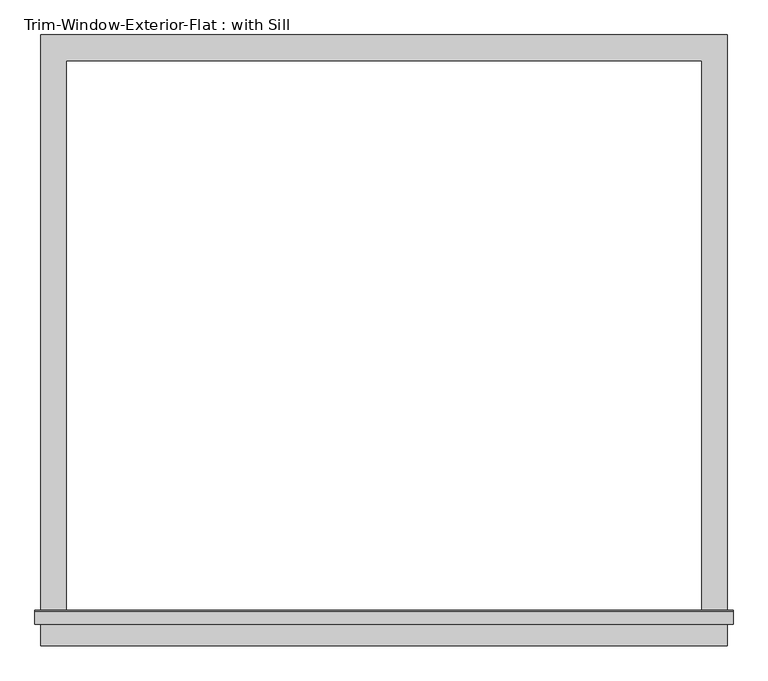
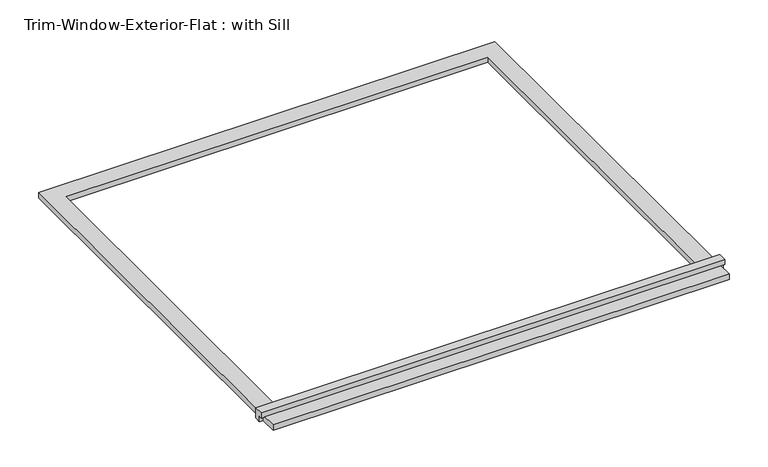
"""IFC4 building model written with IfcOpenShell, lengths in millimetres: proxy geometry, Trim-Window-Exterior-Flat : with Sill."""

from ifc_helpers import new_model, si_unit, frame, origin, origin_with_axes, place, context, project, spatial, polyline, outline, extrude, source, transform, mapped, element, save


def trim_window_exterior_flat_with_sill_cb7cc766(model_context):
    return source(origin(), model_context, "Body", "SweptSolid", [
        extrude(outline(polyline([(762.0, -1241.3823709), (762.0, -1298.5323709), (-762.0, -1298.5323709), (-762.0, -1241.3823709), (762.0, -1241.3823709)])), origin_with_axes(), (0.0, 0.0, 1.0), 19.05),
        extrude(outline(polyline([(-1250.95, 38.1), (-1221.6580645, 38.1), (-1219.2, 19.05), (-1219.2, 0.0), (-1241.3823709, 0.0), (-1241.3823709, 19.05), (-1250.95, 19.05), (-1250.95, 38.1)])), frame((-774.7, 0.0, 0.0), z_axis=(1.0, 0.0, 0.0), x_axis=(0.0, 1.0, 0.0)), (0.0, 0.0, 1.0), 1549.4),
        extrude(outline(polyline([(-762.0, 57.15), (762.0, 57.15), (762.0, -1219.2), (704.85, -1219.2), (704.85, 0.0), (-704.85, 0.0), (-704.85, -1219.2), (-762.0, -1219.2), (-762.0, 57.15)])), origin_with_axes(), (0.0, 0.0, 1.0), 19.05),
    ])


if __name__ == "__main__":
    model = new_model("IFC4")
    model_context = context("Model", 3, world=origin())
    ifc_project = project(units=[si_unit("LENGTHUNIT", "METRE", prefix="MILLI")], contexts=[model_context])
    site = spatial("IfcSite", under=ifc_project)
    building = spatial("IfcBuilding", under=site)
    placement = place(None, origin())
    trim_window_exterior_flat_with_sill_shape = trim_window_exterior_flat_with_sill_cb7cc766(model_context)
    element("IfcBuildingElementProxy", 1, Name="Trim-Window-Exterior-Flat : with Sill", ObjectType="Trim-Window-Exterior-Flat : with Sill", at=placement, inside=building, context=model_context, shape_type="MappedRepresentation", body=[
        mapped(trim_window_exterior_flat_with_sill_shape, transform((0.0, 0.0, 0.0), x_axis=(1.0, 0.0, 0.0), y_axis=(0.0, 1.0, 0.0), z_axis=(0.0, 0.0, 1.0))),
    ])
    save(model, "model.ifc")

# Revit data of these elements
# Type "Trim-Window-Exterior-Flat : with Sill"
#   Trim Width = 0' - 2 1/4"
#   Trim Thickness_Picture Frame = 0' - 1 1/4"
#   Trim Thickness_with Sill = 0' - 0 3/4"
#   Sill Thickness = 0' - 1 1/4"
#   Opening Width [instance default] = 2' - 0"
#   Opening Height [instance default] = 3' - 0"
#   Default Elevation = 4' - 0"
#   Sill = yes
#   Picture Frame = no
#   Trim Material [instance default] = none
# Element 1 (IfcBuildingElementProxy, "Trim-Window-Exterior-Flat : with Sill")
#   Opening Width = 4' - 7 1/2"
#   Opening Height = 4' - 0"
#   Trim Material = Clad - White
#   Materials on its faces: "Clad - White"
# Materials
#   "Clad - White": class "Wood", colour RGB 242 242 238, transparency 0, Cost = 0
